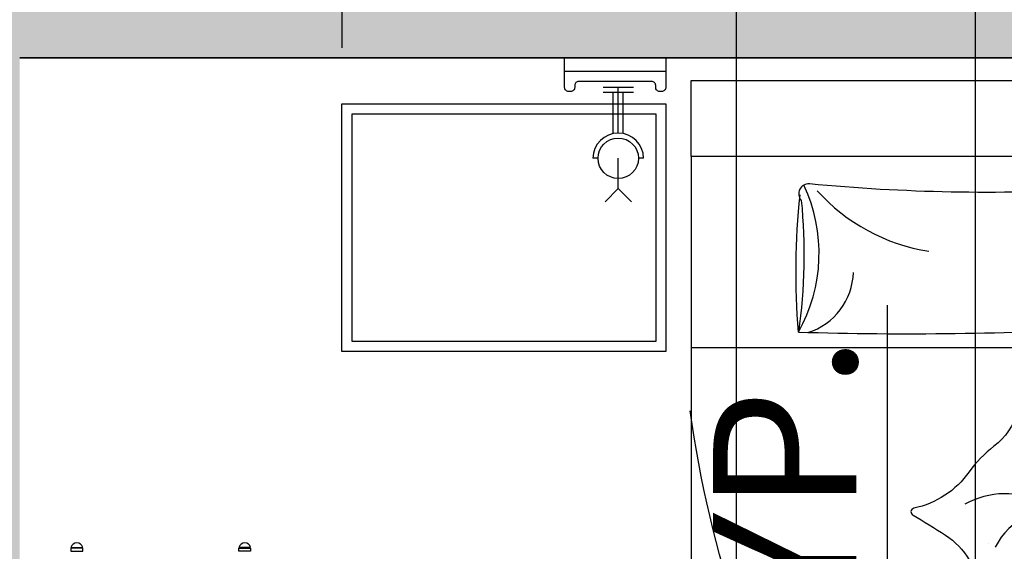
# Model space of a CAD drawing. Units: inches. Extents: x 3592 to 4861, y 1650 to 2243.
# Tile 22 of 30: x 4047 to 4109, y 2125 to 2159. Entities that reach past the tile are written whole.
import ezdxf

# ---------------------------------------------------------------- set-up
doc = ezdxf.new("R2010")
doc.units = ezdxf.units.IN
for name, color, linetype, lineweight in [('A-ANNO-DIMS', 2, 'Continuous', 13), ('A-FURN', 9, 'Continuous', 13), ('A-WALL', 7, 'Continuous', 35), ('estofado', 7, 'Continuous', 25)]:
    doc.layers.add(name, color=color, linetype=linetype, lineweight=lineweight)
doc.layers.add('A-WALL-PATT', color=252, linetype='Continuous', lineweight=13, true_color=0x939598)
for name, color, linetype in [('CEIL', 4, 'Continuous'), ('ELEC', 4, 'Continuous'), ('FUR', 42, 'Continuous'), ('wood', 26, 'Continuous')]:
    doc.layers.add(name, color=color, linetype=linetype)
doc.styles.get("Standard").update_dxf_attribs({"font": 'arial.ttf'})
doc.dimstyles.new('ISO-25', dxfattribs={"dimtxt": 9, "dimasz": 2.5, "dimexe": 1.25, "dimexo": 0.625, "dimtad": 1, "dimlunit": 3, "dimtxsty": 'Standard', "dimcen": 2.5, "dimadec": 0, "dimazin": 0, "dimtfac": 1, "dimtmove": 0, "dimatfit": 3, "dimfxl": 1, "dimarcsym": 0})

# ---------------------------------------------------------------- blocks, each defined once
blk = doc.blocks.new('*X20')
at = {"color": 0}
for p, q in [((3155.9, 8182.9), (3155.9, 8182.9)), ((3147.8, 8143.4), (3147.8, 8143.4)), ((3283, 8049.6), (3283, 8049.6)), ((3209.5, 8023.9), (3209.5, 8023.9)), ((3251.6, 7997), (3251.6, 7997)), ((3154.1, 7950.7), (3154.1, 7950.7))]:
    blk.add_line(p, q, dxfattribs=at)
blk = doc.blocks.new('*X19')
at = {"color": 0}
for p, q in [((3155.9, 8182.9), (3155.9, 8182.9)), ((3139.8, 7939.7), (3139.8, 7939.7))]:
    blk.add_line(p, q, dxfattribs=at)
blk = doc.blocks.new('*X18')
at = {"color": 0}
for p, q in [((3155.9, 8182.9), (3155.9, 8182.9)), ((3139.8, 7939.7), (3139.8, 7939.7))]:
    blk.add_line(p, q, dxfattribs=at)
blk = doc.blocks.new('*X17')
at = {"color": 0}
for p, q in [((3163, 7776.2), (3163, 7776.2)), ((3422.2, 7761.3), (3422.2, 7761.3)), ((3244.3, 7698.6), (3244.3, 7698.6)), ((3340.3, 7689.4), (3340.3, 7689.4)), ((3236.2, 7675.7), (3236.2, 7675.7))]:
    blk.add_line(p, q, dxfattribs=at)
blk = doc.blocks.new('BED1')
for p, q in [((0, -1000), (0, 800)), ((150, 800), (0, 800)), ((150, 800), (150, -1000)), ((2058.7, 800), (150, 800)), ((528, 800), (528, -1000)), ((211.8, 614.9), (277.5, 585.4)), ((2537.2, 404.9), (2237.2, 404.9)), ((2187.2, 354.9), (2187.2, -545.1)), ((2587.2, -545.1), (2587.2, 354.9)), ((2566.3, 178.5), (2565.2, 177.4)), ((2582, 188.1), (2565.4, 174.8)), ((2565.4, 174.8), (2585.7, 165.4)), ((2582, -287.1), (2565.4, -300.5)), ((2566.3, -296.8), (2565.2, -297.9)), ((2565.4, -300.5), (2585.7, -309.9)), ((2237.2, -595.1), (2537.2, -595.1)), ((150, -1000), (0, -1000)), ((150, -1000), (2063.5, -1000))]:
    blk.add_line(p, q)
for points in [[(934, 797.9), (930.9, 797.7), (928.3, 797.4), (926.3, 796.9), (924.9, 796.3), (923.8, 795.6), (923.1, 794.8), (922.7, 793.8), (922.5, 792.7), (922.4, 791.5), (922.5, 790.3), (922.6, 789.2), (922.6, 788.3), (922.6, 787.6), (922.4, 787.3), (922, 787.4), (921.4, 787.9), (920.6, 788.9), (919.5, 790.2), (918.4, 791.6), (917.1, 793.1), (915.9, 794.6), (914.6, 796), (913.3, 797.1), (912.2, 797.9), (911.1, 798.3), (910.1, 798.4), (909.2, 798), (908.3, 797.1), (907.5, 795.8), (906.8, 793.9), (906, 791.4), (905.4, 788.5), (904.8, 785.2), (904.2, 781.7), (903.7, 778.4), (903.2, 775.4), (902.8, 772.9), (902.5, 771.3), (902.3, 770.6), (902.1, 771.2), (902, 772.8), (901.8, 775.2), (901.7, 778.1), (901.5, 781.5), (901.2, 785), (900.8, 788.4), (900.2, 791.5), (899.5, 794.1), (898.6, 796.2), (897.6, 797.9), (896.5, 799.2), (895.3, 800), (894.1, 800.5), (893, 800.7), (891.9, 800.5), (890.9, 800.1), (890, 799), (889.1, 797.1), (888.3, 794), (887.6, 789.3), (886.9, 782.9), (886.2, 774.2), (885.5, 763.1), (884.8, 749.5), (884.2, 734.2), (883.6, 718.3), (883, 702.8), (882.5, 688.8), (882, 677.5), (881.7, 669.8), (881.5, 666.9), (881.3, 669.4), (881.3, 676.7), (881.3, 687.8), (881.2, 701.5), (881.1, 716.8), (880.8, 732.6), (880.2, 748), (879.4, 761.8), (878.3, 773.2), (876.9, 782.2), (875.1, 789.2), (872.9, 794.4), (870.3, 798), (869, 799)], [(2150, -913.5), (2150, 723.2)], [(2327.6, 182.3), (2530, 185.9), (2550.8, 181.9), (2561.7, 179), (2566, 176.7), (2566.9, 174.4), (2566.3, 171.9), (2562, 169.2), (2550.3, 166.5), (2527.7, 163.9), (2490.6, 161.8), (2345.5, 160.2), (2317.8, 158.5)], [(494.7, 3.1), (458.9, 95.3)], [(2149.7, -259.9), (2150, -268.4), (2150.1, -274.1), (2150.1, -278.1), (2150, -281.4), (2149.8, -284), (2149.5, -286.1), (2149.1, -287.8), (2148.7, -289), (2148.1, -289.9), (2147.4, -290.5), (2146.6, -290.8), (2145.6, -291), (2144.6, -291), (2143.6, -291), (2142.7, -290.9), (2141.9, -290.9), (2141.4, -290.9), (2141.1, -291), (2141.2, -291.4), (2141.7, -291.9), (2142.5, -292.6), (2143.5, -293.4), (2144.7, -294.4), (2146, -295.4), (2147.2, -296.5), (2148.4, -297.6), (2149.3, -298.6), (2150, -299.6), (2150.3, -300.5), (2150.4, -301.3), (2150, -302.1), (2149.3, -302.8), (2148.2, -303.5), (2146.6, -304.1), (2144.6, -304.7), (2142.1, -305.2), (2139.3, -305.7), (2136.5, -306.2), (2133.7, -306.6), (2131.2, -307), (2129.2, -307.3), (2127.8, -307.6), (2127.3, -307.8), (2127.7, -308), (2129, -308.1), (2131, -308.2), (2133.5, -308.3), (2136.3, -308.5), (2139.2, -308.7), (2142, -309), (2144.6, -309.5), (2146.8, -310.1), (2148.6, -310.9), (2150, -311.7), (2151, -312.7), (2151.7, -313.6), (2152.1, -314.6), (2152.3, -315.6), (2152.2, -316.5), (2151.8, -317.3), (2150.9, -318.1), (2149.3, -318.8), (2146.7, -319.4), (2142.8, -320), (2137.4, -320.6), (2130.2, -321.2), (2121, -321.8), (2109.7, -322.3), (2096.9, -322.9), (2083.6, -323.4), (2070.7, -323.9), (2059.1, -324.3), (2049.6, -324.7), (2043.2, -325), (2040.8, -325.2), (2042.9, -325.3), (2049, -325.3), (2058.2, -325.3), (2069.6, -325.4), (2082.3, -325.5), (2095.6, -325.8), (2108.4, -326.2), (2119.9, -326.8), (2129.4, -327.8), (2136.9, -329), (2142.7, -330.5), (2147, -332.3), (2150, -334.4), (2150.9, -335.6)], [(2246.5, -294.4), (2530, -289.4), (2550.8, -293.4), (2561.7, -296.3), (2566, -298.6), (2566.9, -300.8), (2566.3, -303.4), (2562, -306.1), (2550.3, -308.8), (2527.7, -311.3), (2490.6, -313.5), (2345.5, -315), (2238.6, -321.8)], [(1733.7, -998.3), (1731.1, -998.1), (1729, -997.8), (1727.4, -997.4), (1726.1, -997), (1725.2, -996.4), (1724.7, -995.7), (1724.3, -994.8), (1724.1, -993.9), (1724.1, -992.9), (1724.1, -991.9), (1724.2, -991), (1724.2, -990.2), (1724.2, -989.7), (1724.1, -989.4), (1723.8, -989.5), (1723.2, -990), (1722.5, -990.8), (1721.7, -991.8), (1720.7, -993), (1719.7, -994.3), (1718.6, -995.5), (1717.5, -996.6), (1716.5, -997.6), (1715.5, -998.3), (1714.6, -998.6), (1713.8, -998.6), (1713, -998.3), (1712.3, -997.6), (1711.7, -996.5), (1711, -994.9), (1710.4, -992.9), (1709.9, -990.4), (1709.4, -987.6), (1708.9, -984.8), (1708.5, -982), (1708.1, -979.5), (1707.8, -977.4), (1707.5, -976.1), (1707.3, -975.5), (1707.1, -976), (1707, -977.3), (1706.9, -979.3), (1706.8, -981.8), (1706.7, -984.6), (1706.4, -987.5), (1706.1, -990.3), (1705.6, -992.9), (1705, -995.1), (1704.2, -996.9), (1703.4, -998.3), (1702.4, -999.3), (1701.5, -1000), (1700.5, -1000.4), (1699.6, -1000.6), (1698.7, -1000.4), (1697.8, -1000.1), (1697, -999.2), (1696.3, -997.6), (1695.7, -995), (1695.1, -991.1), (1694.5, -985.7), (1693.9, -978.5), (1693.3, -969.3), (1692.8, -957.9), (1692.2, -945.2), (1691.7, -931.9), (1691.2, -919), (1690.8, -907.4), (1690.4, -897.9), (1690.1, -891.5), (1689.9, -889.1), (1689.8, -891.2), (1689.8, -897.3), (1689.8, -906.5), (1689.7, -917.9), (1689.6, -930.6), (1689.4, -943.8), (1688.9, -956.6), (1688.3, -968.1), (1687.3, -977.6), (1686.1, -985.2), (1684.6, -991), (1682.8, -995.3), (1680.7, -998.3), (1679.6, -999.2)]]:
    blk.add_lwpolyline(points)
for points in [[(489.2, 619.6, 0.144019), (207.6, 617.9, 0.248643)], [(205.5, 619.6, 0.267769), (215.1, 582.4, -0.037739), (204.3, 21.8, 0.684696), (236.7, 5.5, -0.060702), (497.2, 0.1, -0.046649), (225.9, 3.1, -1.318436)], [(497.2, 0.1, 0.021276), (489.2, 619.6, -0.206383), (326.6, 509.4, 0.237198)], [(211.8, 12.8, 0.143972), (361.6, 262.9, 1.292232)], [(886.4, -150, -0.069098), (985, -66.5, 0.658965), (982.1, -48.7, -0.049789), (927.4, -29, -0.103757), (896.6, -5.4, 0.055725), (800.9, 83.3, -0.11866), (782.7, 104.9, 0.016811), (761.6, 143.9, 0.70791), (748.3, 144, -0.16964), (551.9, -96.6, 0.664036), (554, -110.7, 0.023706), (627, -144.7, -0.134834), (683.2, -188, 0.012748), (746.3, -267.4)], [(969.1, -259.1, 0.263265), (936.3, -236.9, -0.026108), (909.2, -233.2, 0.027613), (945.1, -234.2, -0.089259), (872.7, -120, 0.662242), (857.6, -119.3, -0.162037), (651.8, -332.7, 0.676499), (654, -354.5, -0.160513), (722.9, -401.5, 0.07473), (773.5, -450.3, -0.187721), (845.5, -559.9, 0.70791), (858.8, -561.4, -0.010003), (898.6, -497.3, -0.113819), (947.3, -450.2, 0.099539), (1032.5, -372.4, -0.173425), (1070.9, -346.4, 0.589988), (1076.2, -326.1, 0.137312), (923.9, -245.9, 0.137312)], [(489.2, -168.2, 0.144019), (207.6, -169.9, 0.248643)], [(205.5, -168.2, 0.267769), (215.1, -205.4, -0.037739), (204.3, -766, 0.684696), (236.7, -782.3, -0.060702), (497.2, -787.7, -0.046649), (225.9, -784.7, -1.318436)], [(497.2, -787.7, 0.021276), (489.2, -168.2, -0.206383), (326.6, -278.4, 0.237198)], [(1446, -733.4, -0.095039), (652.8, -1001.7)]]:
    blk.add_lwpolyline(points, format="xyb")
for centre, radius, start, end in [((3208.8, 1363.3), 2739.4, 191.8679, 206.3247), ((2062.7, 713.7), 86.5, 0, 93.5376), ((1608.1, 842.5), 496.3, 305.1901, 354.0206), ((1138.6, 793.9), 983.2, 294.6078, 358.3033), ((2237.2, 354.9), 50, 90, 180), ((2321.1, 409.7), 84.5, 185.6196, 217.1396), ((2227.5, 373.5), 32.8, 17.833, 72.8005), ((2546.9, 373.5), 32.8, 107.1995, 162.167), ((2453.3, 409.7), 84.5, 322.8604, 354.3804), ((2537.2, 354.9), 50, 0, 90), ((2098.7, 754.7), 1625, 193.905, 207.8169), ((2201.9, 323.3), 34.8, 50.8413, 114.9586), ((2212.2, 381.5), 36.5, 226.8095, 258.3841), ((2572.5, 323.3), 34.8, 65.0414, 129.1587), ((2562.2, 381.5), 36.5, 281.6159, 313.1905), ((751.8, 88.7), 34.9, 336.8352, 27.7218), ((684.2, 86), 100.3, 353.675, 10.882), ((1074.1, 198.8), 306.1, 197.8602, 241.5122), ((341.4, -277.7), 318.5, 60.7125, 115.009), ((978.5, -68.6), 14.3, 39.7097, 85.9506), ((983.7, -79.5), 20.8, 73.7967, 130.4566), ((602.5, -324), 198.6, 43.2035, 95.0556), ((3208.8, 1363.3), 2739.4, 212.9314, 216.951), ((981.1, -281.8), 131.1, 164.0372, 243.4536), ((980, -379), 163.4, 152.6104, 209.361), ((3208.8, 1363.3), 2739.4, 218.6329, 229.9449), ((2098.7, 754.7), 1625, 226.5887, 246.3156), ((3402.5, -342.9), 1408.5, 182.9917, 205.6819), ((2188.1, -476.2), 73, 269.4513, 322.8027), ((-34.4, -471.2), 376.5, 312.0118, 350.9635), ((2178, -513.5), 33, 286.1827, 338.1386), ((2572.5, -513.6), 34.8, 230.8413, 294.9586), ((2562.2, -571.8), 36.5, 46.8095, 78.3841), ((2237.2, -545.1), 50, 180, 270), ((2271.1, -580.9), 35.8, 148.9055, 197.5541), ((2453.3, -600), 84.5, 5.6196, 37.1396), ((2537.2, -545.1), 50, 270, 0), ((2546.9, -563.8), 32.8, 197.833, 252.8005), ((375.7, -807.4), 128.2, 17.4073, 88.5129), ((341.4, -1065.5), 318.5, 60.7125, 115.009), ((1929.1, -1126), 250.5, 37.8553, 88.4405), ((2063.5, -913.5), 86.5, 270, 0)]:
    blk.add_arc(centre, radius, start, end)
for name in ['*X19', '*X18', '*X20', '*X17']:
    blk.add_blockref(name, (-2425.3, -8101.4))
blk = doc.blocks.new('APLIQ')
at = {"layer": 'ELEC'}
for p, q in [((0, 0.2), (-0.0261, 0.2261)), ((0, 0.2), (0.0261, 0.2261)), ((0, 0.2), (0, 0.14)), ((-0.05, 0.14), (-0.04, 0.14)), ((0.04, 0.14), (0.05, 0.14)), ((-0.01, 0.09), (-0.01, 0.01)), ((0, 0.09), (0, 0)), ((0.01, 0.09), (0.01, 0.01)), ((-0.03, 0.01), (0.03, 0.01)), ((-0.03, 0), (0.03, 0))]:
    blk.add_line(p, q, dxfattribs=at)
blk.add_circle((0, 0.14), 0.04, dxfattribs=at)
blk.add_arc((0, 0.14), 0.05, 180, 0, dxfattribs=at)
blk = doc.blocks.new('A$C68AE1801')
at = {"layer": 'FUR'}
for points in [[(2.5416, 3.18), (2.5416, 2.54), (2.0516, 2.54), (2.0516, 3.18)], [(2.5216, 3.16), (2.5216, 2.56), (2.0716, 2.56), (2.0716, 3.16)]]:
    blk.add_lwpolyline(points, close=True, dxfattribs=at)
at = {"layer": 'wood'}
blk.add_line((2.6057, 2.74), (2.6057, 2.54), dxfattribs=at)
blk.add_lwpolyline([(2.5657, 2.728), (2.5657, 2.732, -0.414214), (2.5737, 2.74), (2.6321, 2.74), (2.6321, 2.54), (2.5737, 2.54, -0.414214), (2.5657, 2.548), (2.5657, 2.552, -0.414214), (2.5737, 2.56), (2.5777, 2.56, 0.414214), (2.5857, 2.568), (2.5857, 2.712, 0.414214), (2.5777, 2.72), (2.5737, 2.72, -0.414214)], format="xyb", close=True, dxfattribs=at)
at = {"layer": 'CEIL', "rotation": 90}
blk.add_blockref('APLIQ', (2.5736, 2.634), dxfattribs=at)
at = {"layer": 'FUR', "xscale": 0.001, "yscale": 0.001, "zscale": 0.001, "rotation": 180}
blk.add_blockref('BED1', (2.5872, 1.49), dxfattribs=at)
blk = doc.blocks.new('Aparador Aido WV')
at = {"layer": 'estofado', "ltscale": 0.5}
for p, q in [((-0.9067, -0.0817), (-0.9067, -0.1006)), ((-0.9067, -0.3683), (-0.9067, -0.3494))]:
    blk.add_line(p, q, dxfattribs=at)
for points in [[(-0.9054, -0.0817), (-0.9009, -0.0817), (-0.9009, -0.1006), (-0.9054, -0.1006)], [(-0.9054, -0.3683), (-0.9009, -0.3683), (-0.9009, -0.3494), (-0.9054, -0.3494)]]:
    blk.add_lwpolyline(points, close=True, dxfattribs=at)
for centre in [(-0.904, -0.0911), (-0.904, -0.3589)]:
    blk.add_arc(centre, 0.0098, 105.9849, 254.0151, dxfattribs=at)
blk = doc.blocks.new('*D150')
at = {"layer": 'A-ANNO-DIMS', "color": 0, "lineweight": -2, "transparency": 16777216}
for p, q in [((4101.85, 2020.278), (4101.85, 2140.684)), ((4100.037, 2020.278), (4103.1, 2020.278)), ((4101.85, 2006.522), (4101.85, 2017.778)), ((4100.037, 2004.022), (4103.1, 2004.022))]:
    blk.add_line(p, q, dxfattribs=at)
at = {"layer": 'A-ANNO-DIMS', "color": 0, "transparency": 16777216}
for points in [[(4101.433, 2017.778), (4102.267, 2017.778), (4101.85, 2020.278)], [(4101.433, 2006.522), (4102.267, 2006.522), (4101.85, 2004.022)]]:
    blk.add_solid(points, dxfattribs=at)
at = {"layer": 'Defpoints', "color": 0, "transparency": 16777216}
for p in [(4099.412, 2020.278), (4101.85, 2020.278), (4099.412, 2004.022)]:
    blk.add_point(p, dxfattribs=at)
at = {"layer": 'A-ANNO-DIMS', "color": 0, "transparency": 16777216, "insert": (4096.571, 2081.731), "char_height": 9, "attachment_point": 5, "rotation": 90}
blk.add_mtext('BASIN 1\'-4 1/2" TYP.', dxfattribs=at)
blk = doc.blocks.new('*D154')
at = {"layer": 'A-ANNO-DIMS', "color": 0, "lineweight": -2, "transparency": 16777216}
for p, q in [((4067.606, 2156.844), (4067.606, 2172.621)), ((4168.621, 2156.844), (4168.621, 2172.621)), ((4067.606, 2171.371), (3930.452, 2171.371)), ((4166.121, 2171.371), (4070.106, 2171.371))]:
    blk.add_line(p, q, dxfattribs=at)
at = {"layer": 'A-ANNO-DIMS', "color": 0, "transparency": 16777216}
for points in [[(4070.106, 2171.788), (4070.106, 2170.955), (4067.606, 2171.371)], [(4166.121, 2171.788), (4166.121, 2170.955), (4168.621, 2171.371)]]:
    blk.add_solid(points, dxfattribs=at)
at = {"layer": 'Defpoints', "color": 0, "transparency": 16777216}
for p in [(4067.606, 2171.371), (4067.606, 2156.219), (4168.621, 2156.219)]:
    blk.add_point(p, dxfattribs=at)
at = {"layer": 'A-ANNO-DIMS', "color": 0, "transparency": 16777216, "insert": (3997.779, 2176.653), "char_height": 9, "attachment_point": 5}
blk.add_mtext('BED GROUP 8\'-5" TYP.', dxfattribs=at)
blk = doc.blocks.new('*D179')
at = {"layer": 'A-ANNO-DIMS', "color": 0, "lineweight": -2, "transparency": 16777216}
for p, q in [((4092.37, 2010.809), (4092.37, 2193.519)), ((4107.37, 2020.844), (4107.37, 2193.519)), ((4094.87, 2192.269), (4104.87, 2192.269)), ((4107.37, 2192.269), (4134.197, 2192.269))]:
    blk.add_line(p, q, dxfattribs=at)
at = {"layer": 'A-ANNO-DIMS', "color": 0, "transparency": 16777216}
for points in [[(4094.87, 2192.686), (4094.87, 2191.852), (4092.37, 2192.269)], [(4104.87, 2192.686), (4104.87, 2191.852), (4107.37, 2192.269)]]:
    blk.add_solid(points, dxfattribs=at)
at = {"layer": 'Defpoints', "color": 0, "transparency": 16777216}
for p in [(4107.37, 2192.269), (4107.37, 2020.219), (4092.37, 2010.184)]:
    blk.add_point(p, dxfattribs=at)
at = {"layer": 'A-ANNO-DIMS', "color": 0, "transparency": 16777216, "insert": (4122.033, 2197.492), "char_height": 9, "attachment_point": 5}
blk.add_mtext('1\'-3"', dxfattribs=at)

msp = doc.modelspace()

# ---------------------------------------------------------------- hatches: boundary and pattern name
at = {"layer": 'A-WALL-PATT'}
h = msp.add_hatch(color=256, dxfattribs=at)
h.dxf.hatch_style = 1
h.paths.add_polyline_path([(4398.37, 2165.219), (4038.37, 2165.219), (4038.37, 1993.219), (4047.37, 1993.219), (4047.37, 2156.219), (4191.37, 2156.219), (4191.37, 2150.219), (4195.37, 2150.219), (4195.37, 2156.219), (4256.37, 2156.219), (4256.37, 2150.219), (4265.37, 2150.219), (4265.37, 2156.219), (4389.37, 2156.219), (4389.37, 2114.219), (4398.37, 2114.219)])
h.paths.add_polyline_path([(4265.37, 2102.219), (4256.37, 2102.219), (4256.37, 2096.219), (4195.37, 2096.219), (4195.37, 2102.219), (4191.37, 2102.219), (4191.37, 2020.219), (4195.37, 2020.219), (4195.37, 2087.219), (4256.37, 2087.219), (4256.37, 2020.219), (4306.37, 2020.219), (4306.37, 2024.219), (4265.37, 2024.219)], flags=17)
h.paths.add_polyline_path([(4398.37, 2066.219), (4389.37, 2066.219), (4389.37, 2024.219), (4348.37, 2024.219), (4348.37, 2020.219), (4389.37, 2020.219), (4389.37, 1989.719), (4398.37, 1989.719)])
h.paths.add_polyline_path([(4398.37, 1941.719), (4389.37, 1941.719), (4389.37, 1911.219), (4301.37, 1911.219), (4301.37, 1907.219), (4389.37, 1907.219), (4389.37, 1865.219), (4398.37, 1865.219)])
h.paths.add_polyline_path([(4398.37, 1817.219), (4389.37, 1817.219), (4389.37, 1775.219), (4265.37, 1775.219), (4265.37, 1911.219), (4256.37, 1911.219), (4256.37, 1817.219), (4220.87, 1817.219), (4220.87, 1808.219), (4256.37, 1808.219), (4256.37, 1766.219), (4389.37, 1766.219), (4389.37, 1694.219), (4256.37, 1694.219), (4256.37, 1685.219), (4398.37, 1685.219)])
h.paths.add_polyline_path([(4178.87, 1817.219), (4077.37, 1817.219), (4077.37, 1808.219), (4178.87, 1808.219)])
h.paths.add_polyline_path([(4111.37, 2020.219), (4155.37, 2020.219), (4155.37, 2024.219), (4077.37, 2024.219), (4077.37, 2020.219), (4107.37, 2020.219), (4107.37, 1942.219), (4047.37, 1942.219), (4047.37, 1969.219), (4038.37, 1969.219), (4038.37, 1911.219), (4047.37, 1911.219), (4047.37, 1938.219), (4107.37, 1938.219), (4107.37, 1860.219), (4077.37, 1860.219), (4077.37, 1856.219), (4111.37, 1856.219)])
h.paths.add_polyline_path([(4047.37, 1887.219), (4038.37, 1887.219), (4038.37, 1685.219), (4152.37, 1685.219), (4152.37, 1715.219), (4143.37, 1715.219), (4143.37, 1694.219), (4047.37, 1694.219)])
h.paths.add_polyline_path([(4152.37, 1772.219), (4143.37, 1772.219), (4143.37, 1751.219), (4152.37, 1751.219)], flags=17)

# ---------------------------------------------------------------- linework, layer by layer
at = {"layer": 'A-WALL'}
msp.add_line((4047.37, 2156.219), (4191.37, 2156.219), dxfattribs=at)

# ---------------------------------------------------------------- block references
at = {"layer": 'A-FURN'}
for name, p, xscale, yscale, zscale, rotation in [('A$C68AE1801', (4168.621, 2072.607), 31.7658940618111, 31.7658940618111, 31.7658940618111, 90), ('Aparador Aido WV', (4065.086, 2089.784), 39.3701, 39.3701, 39.3701, 270)]:
    msp.add_blockref(name, p, dxfattribs=dict(at, xscale=xscale, yscale=yscale, zscale=zscale, rotation=rotation))

# ---------------------------------------------------------------- dimensions: what is measured, and where the dimension line sits
at = {"layer": 'A-ANNO-DIMS'}
for base, p1, p2, angle, text, picture, middle in [((4067.606, 2171.371), (4168.621, 2156.219), (4067.606, 2156.219), 180, 'BED GROUP <> TYP.', '*D154', (3997.779, 2176.653)), ((4101.85, 2020.278), (4099.412, 2004.022), (4099.412, 2020.278), 90, 'BASIN <> TYP.', '*D150', (4096.571, 2081.731))]:
    dim = msp.add_linear_dim(base=base, p1=p1, p2=p2, angle=angle, text=text, dimstyle='ISO-25', override={"dimdec": 1, "dimlfac": 1, "dimrnd": 0, "dimzin": 1, "dimdsep": 46, "dimlunit": 4, "dimfrac": 2}, dxfattribs=at)
    dim.commit()
    dim.dimension.update_dxf_attribs({"geometry": picture, "text_midpoint": middle})
dim = msp.add_linear_dim(base=(4107.37, 2192.269), p1=(4092.37, 2010.184), p2=(4107.37, 2020.219), dimstyle='ISO-25', override={"dimdec": 1, "dimlfac": 1, "dimrnd": 0, "dimzin": 1, "dimdsep": 46, "dimlunit": 4, "dimfrac": 2}, dxfattribs=at)
dim.commit()
dim.dimension.update_dxf_attribs({"geometry": '*D179', "text_midpoint": (4122.033, 2197.492)})

doc.saveas('drawing.dxf')
